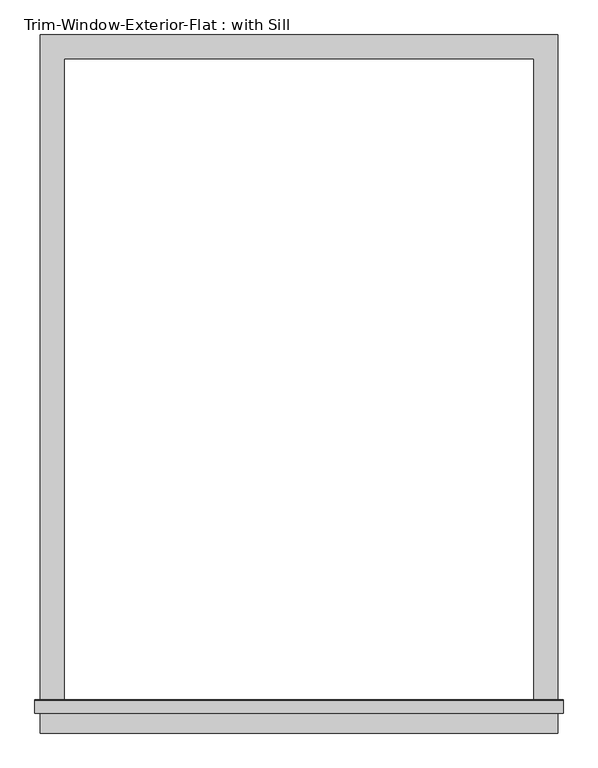
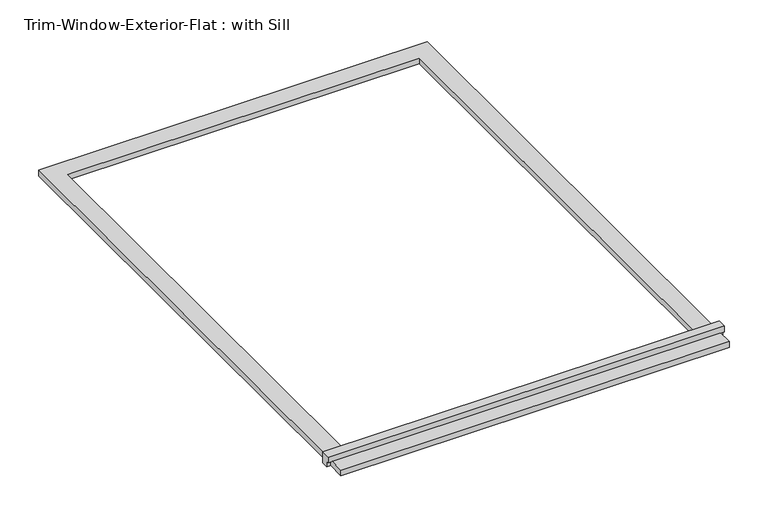
"""IFC4 building model written with IfcOpenShell, lengths in millimetres: proxy geometry, Trim-Window-Exterior-Flat : with Sill."""

from ifc_helpers import new_model, si_unit, frame, origin, origin_with_axes, place, context, project, spatial, polyline, outline, extrude, source, transform, mapped, element, save


def trim_window_exterior_flat_with_sill_dc35da0b(model_context):
    return source(origin(), model_context, "Body", "SweptSolid", [
        extrude(outline(polyline([(615.95, -1546.1823709), (615.95, -1603.3323709), (-615.95, -1603.3323709), (-615.95, -1546.1823709), (615.95, -1546.1823709)])), origin_with_axes(), (0.0, 0.0, 1.0), 19.05),
        extrude(outline(polyline([(-1555.75, 38.1), (-1526.4580645, 38.1), (-1524.0, 19.05), (-1524.0, 0.0), (-1546.1823709, 0.0), (-1546.1823709, 19.05), (-1555.75, 19.05), (-1555.75, 38.1)])), frame((-628.65, 0.0, 0.0), z_axis=(1.0, 0.0, 0.0), x_axis=(0.0, 1.0, 0.0)), (0.0, 0.0, 1.0), 1257.3),
        extrude(outline(polyline([(-615.95, 57.15), (615.95, 57.15), (615.95, -1524.0), (558.8, -1524.0), (558.8, 0.0), (-558.8, 0.0), (-558.8, -1524.0), (-615.95, -1524.0), (-615.95, 57.15)])), origin_with_axes(), (0.0, 0.0, 1.0), 19.05),
    ])


if __name__ == "__main__":
    model = new_model("IFC4")
    model_context = context("Model", 3, world=origin())
    ifc_project = project(units=[si_unit("LENGTHUNIT", "METRE", prefix="MILLI")], contexts=[model_context])
    site = spatial("IfcSite", under=ifc_project)
    building = spatial("IfcBuilding", under=site)
    placement = place(None, origin())
    trim_window_exterior_flat_with_sill_shape = trim_window_exterior_flat_with_sill_dc35da0b(model_context)
    element("IfcBuildingElementProxy", 1, Name="Trim-Window-Exterior-Flat : with Sill", ObjectType="Trim-Window-Exterior-Flat : with Sill", at=placement, inside=building, context=model_context, shape_type="MappedRepresentation", body=[
        mapped(trim_window_exterior_flat_with_sill_shape, transform((0.0, 0.0, 0.0), x_axis=(1.0, 0.0, 0.0), y_axis=(0.0, 1.0, 0.0), z_axis=(0.0, 0.0, 1.0))),
    ])
    save(model, "model.ifc")

# Revit data of these elements
# Type "Trim-Window-Exterior-Flat : with Sill"
#   Trim Width = 0' - 2 1/4"
#   Trim Thickness_Picture Frame = 0' - 1 1/4"
#   Trim Thickness_with Sill = 0' - 0 3/4"
#   Sill Thickness = 0' - 1 1/4"
#   Opening Width [instance default] = 2' - 0"
#   Opening Height [instance default] = 3' - 0"
#   Default Elevation = 4' - 0"
#   Sill = yes
#   Picture Frame = no
#   Trim Material [instance default] = none
# Element 1 (IfcBuildingElementProxy, "Trim-Window-Exterior-Flat : with Sill")
#   Opening Width = 3' - 8"
#   Opening Height = 5' - 0"
#   Trim Material = Clad - White
#   Materials on its faces: "Clad - White"
# Materials
#   "Clad - White": class "Wood", colour RGB 242 242 238, transparency 0, Cost = 0
